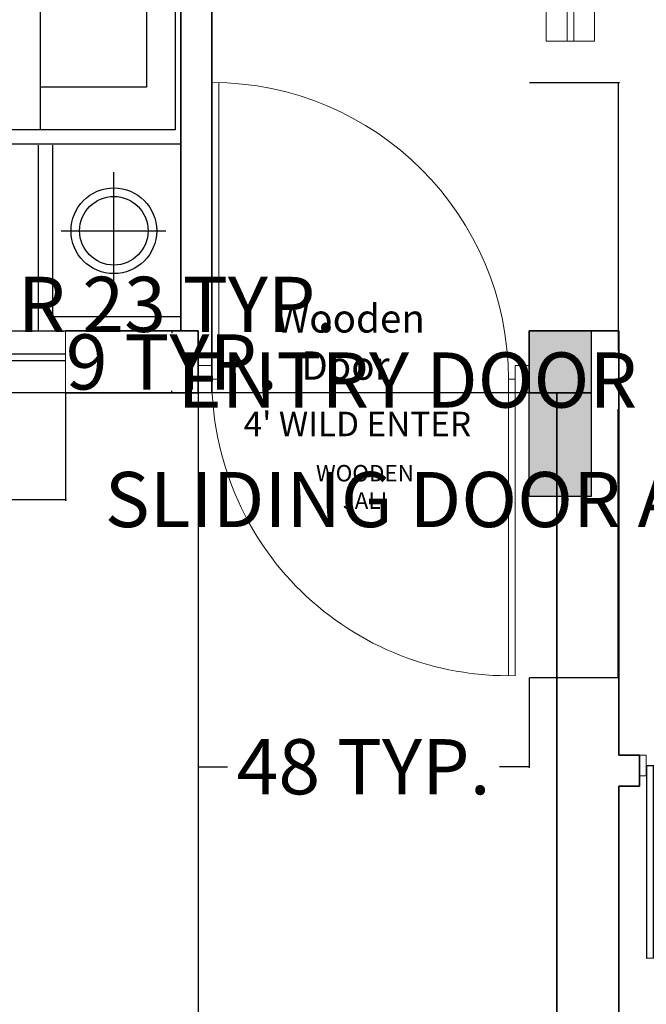
# Model space of a CAD drawing. Units: inches. Extents: x -48 to 50072, y 0 to 21068.
# Tile 61 of 75: x 883 to 974, y 660 to 803. Entities that reach past the tile are written whole.
import ezdxf

# ---------------------------------------------------------------- set-up
doc = ezdxf.new("R2010")
doc.units = ezdxf.units.IN
doc.header["$MEASUREMENT"] = 0
for name, color, linetype, lineweight in [('A-ANNO-DIMS', 2, 'Continuous', 18), ('A-ANNO-TEXT', 7, 'Continuous', 18), ('A-COLS', 1, 'Continuous', 35), ('A-DOOR', 4, 'Continuous', 18), ('A-FLOR-SCRN', 32, 'Continuous', 18), ('A-WALL', 7, 'Continuous', 35), ('FURNITURE', 44, 'Continuous', 18)]:
    doc.layers.add(name, color=color, linetype=linetype, lineweight=lineweight)
doc.layers.add('Layer3', color=176, linetype='Continuous')
doc.styles.get("Standard").update_dxf_attribs({"font": 'arial.ttf'})
doc.dimstyles.get("Standard").update_dxf_attribs({"dimtxt": 8, "dimasz": 0.18, "dimexe": 0.18, "dimexo": 0.0625, "dimgap": 0.09, "dimtad": 0, "dimtih": 1, "dimtoh": 1, "dimdec": 1, "dimzin": 0, "dimdsep": 46, "dimlunit": 4, "dimtxsty": 'Standard', "dimblk": 'ARCHTICK', "dimcen": 0.09, "dimadec": 0, "dimazin": 0, "dimtfac": 1, "dimtdec": 1, "dimtofl": 0, "dimtmove": 0, "dimatfit": 3, "dimldrblk": 'ARCHTICK', "dimfxl": 1, "dimtolj": 1, "dimtzin": 0, "dimarcsym": 0})

# ---------------------------------------------------------------- blocks, each defined once
blk = doc.blocks.new('bnniku')
at = {"layer": 'Defpoints'}
h = blk.add_hatch(color=256, dxfattribs=at)
h.dxf.hatch_style = 1
h.paths.add_polyline_path([(767.55, 1114.04), (758.55, 1114.04), (758.55, 1090.04), (767.55, 1090.04)])
for p, q in [((758.55, 1114.04), (767.55, 1114.04)), ((758.55, 1090.04), (758.55, 1114.04)), ((767.55, 1114.04), (767.55, 1090.04)), ((767.55, 1090.04), (758.55, 1090.04))]:
    blk.add_line(p, q, dxfattribs=at)
blk = doc.blocks.new('fdsghhhhhhygr')
for p, q in [((41.77, 686.77), (41.77, 677.77)), ((144.77, 677.77), (144.77, 686.77))]:
    blk.add_line(p, q)
at = {"layer": 'Defpoints'}
for p, q in [((91.27, 683.47), (144.77, 683.47)), ((91.27, 683.47), (91.27, 682.47)), ((91.27, 682.47), (144.77, 682.47)), ((41.77, 682.07), (95.27, 682.07)), ((41.77, 681.07), (95.27, 681.07)), ((95.27, 682.07), (95.27, 681.07))]:
    blk.add_line(p, q, dxfattribs=at)
at = {"layer": 'Layer3'}
for p, q in [((41.77, 686.77), (144.77, 686.77)), ((144.77, 677.77), (41.77, 677.77))]:
    blk.add_line(p, q, dxfattribs=at)
blk = doc.blocks.new('gthyerhy')
at = {"layer": 'Defpoints'}
for p, q in [((665.59, 603.33), (665.59, 631.33)), ((666.59, 603.33), (666.59, 631.32)), ((665.59, 603.33), (693.59, 603.33))]:
    blk.add_line(p, q, dxfattribs=at)
blk.add_arc((665.59, 603.33), 28, 0, 90, dxfattribs=at)
at = {"insert": (674.82, 600.63), "char_height": 2.3647, "attachment_point": 1}
blk.add_mtext_dynamic_manual_height_columns('\\pxqc;WOODEN ^JDOOR', width=6.8949, gutter_width=11.82, heights=[0], dxfattribs=at)
blk = doc.blocks.new('nhrygfdu7yu')
at = {"layer": 'Defpoints'}
for p, q in [((1019.17, 828.61), (845.97, 828.61)), ((845.97, 801.61), (845.97, 828.61)), ((848.67, 804.31), (848.67, 828.61)), ((881.27, 716.83), (881.27, 828.61)), ((983.87, 828.61), (983.87, 716.83)), ((1016.47, 804.31), (1016.47, 828.61)), ((1019.17, 801.61), (1019.17, 828.61)), ((884.03, 719.53), (884.03, 827.53)), ((884.03, 827.53), (981.17, 827.53)), ((981.17, 827.53), (981.17, 719.53)), ((864.18, 805.04), (864.18, 824.84)), ((1000.24, 805.98), (1000.24, 825.78)), ((892.12, 822.13), (892.12, 801.97)), ((929.67, 822.13), (892.12, 822.13)), ((929.67, 822.13), (929.67, 801.78)), ((935.52, 822.13), (935.52, 801.78)), ((935.52, 822.13), (973.07, 822.13)), ((973.07, 822.13), (973.07, 801.97)), ((926.47, 818.07), (927.21, 812.5)), ((947.88, 818.06), (943.61, 812.45)), ((1010.72, 815.93), (989.15, 815.93)), ((874.65, 814.99), (853.09, 814.99)), ((927.21, 812.5), (925.82, 805.91)), ((934.43, 807.75), (933.36, 812.55)), ((943.61, 812.45), (939.55, 805.41)), ((914.58, 810.18), (913.28, 809.99)), ((919.69, 808.14), (914.58, 810.18)), ((923.4, 803.12), (919.69, 808.14)), ((935.49, 804.66), (934.43, 807.75)), ((881.07, 804.31), (848.67, 804.31)), ((881.07, 804.31), (881.07, 804.31)), ((916.07, 804.42), (910.77, 803.49)), ((919.78, 804.61), (916.07, 804.42)), ((923.4, 803.12), (919.78, 804.61)), ((925.82, 805.91), (923.4, 803.12)), ((938.59, 802.42), (935.49, 804.66)), ((939.55, 805.41), (938.59, 802.42)), ((938.59, 802.42), (945.53, 804.13)), ((945.53, 804.13), (951.08, 803.38)), ((984.07, 804.31), (1016.47, 804.31)), ((984.07, 804.31), (984.07, 804.31)), ((910.77, 803.49), (910.59, 803.15)), ((923.4, 803.12), (925.08, 798.67)), ((923.4, 803.12), (933.44, 802.1)), ((935.45, 803.17), (936.69, 800.13)), ((938.59, 802.42), (937.95, 797.34)), ((938.59, 802.42), (941.26, 799.01)), ((951.08, 803.38), (953.02, 802.3)), ((881.07, 801.61), (845.97, 801.61)), ((884.06, 801.97), (981.18, 801.97)), ((933.44, 802.1), (936.13, 800.15)), ((984.07, 801.61), (1019.17, 801.61)), ((925.08, 798.67), (923.96, 794.21)), ((936.13, 800.15), (936.78, 799.69)), ((936.69, 800.13), (937.65, 797.78)), ((941.26, 799.01), (944.78, 796.45)), ((937.86, 796.54), (937.22, 791.44)), ((944.78, 796.45), (949.8, 796.45)), ((981.13, 793.06), (883.98, 783.7)), ((923.96, 794.21), (921.07, 790.83)), ((906.36, 766.47), (977.44, 792.73)), ((976.41, 779.36), (976.41, 779.36)), ((978.98, 779.36), (978.98, 779.36)), ((962.27, 776.79), (962.27, 776.79)), ((964.84, 776.79), (964.84, 776.79)), ((967.41, 776.79), (967.41, 776.79)), ((969.98, 776.79), (969.98, 776.79)), ((972.55, 776.79), (972.55, 776.79)), ((975.13, 776.79), (975.13, 776.79)), ((977.7, 776.79), (977.7, 776.79)), ((980.27, 776.79), (980.27, 776.79)), ((950.69, 774.21), (950.69, 774.21)), ((953.27, 774.21), (953.27, 774.21)), ((955.84, 774.21), (955.84, 774.21)), ((958.41, 774.21), (958.41, 774.21)), ((960.98, 774.21), (960.98, 774.21)), ((963.55, 774.21), (963.55, 774.21)), ((966.13, 774.21), (966.13, 774.21)), ((968.7, 774.21), (968.7, 774.21)), ((941.69, 771.64), (941.69, 771.64)), ((944.27, 771.64), (944.27, 771.64)), ((946.84, 771.64), (946.84, 771.64)), ((949.41, 771.64), (949.41, 771.64)), ((951.98, 771.64), (951.98, 771.64)), ((954.55, 771.64), (954.55, 771.64)), ((935.26, 769.07), (935.26, 769.07)), ((937.84, 769.07), (937.84, 769.07)), ((940.41, 769.07), (940.41, 769.07)), ((942.98, 769.07), (942.98, 769.07)), ((928.83, 766.5), (928.83, 766.5)), ((931.41, 766.5), (931.41, 766.5)), ((933.98, 766.5), (933.98, 766.5)), ((936.55, 766.5), (936.55, 766.5)), ((975.13, 766.5), (975.13, 766.5)), ((977.7, 766.5), (977.7, 766.5)), ((980.27, 766.5), (980.27, 766.5)), ((924.98, 763.93), (924.98, 763.93)), ((927.55, 763.93), (927.55, 763.93)), ((930.12, 763.93), (930.12, 763.93)), ((963.55, 763.93), (963.55, 763.93)), ((966.13, 763.93), (966.13, 763.93)), ((968.7, 763.93), (968.7, 763.93)), ((971.27, 763.93), (971.27, 763.93)), ((973.84, 763.93), (973.84, 763.93)), ((976.41, 763.93), (976.41, 763.93)), ((978.98, 763.93), (978.98, 763.93)), ((921.12, 761.35), (921.12, 761.35)), ((923.69, 761.35), (923.69, 761.35)), ((954.55, 761.35), (954.55, 761.35)), ((957.12, 761.35), (957.12, 761.35)), ((959.7, 761.35), (959.7, 761.35)), ((962.27, 761.35), (962.27, 761.35)), ((964.84, 761.35), (964.84, 761.35)), ((967.41, 761.35), (967.41, 761.35)), ((969.98, 761.35), (969.98, 761.35)), ((972.55, 761.35), (972.55, 761.35)), ((975.13, 761.35), (975.13, 761.35)), ((917.26, 758.78), (917.26, 758.78)), ((919.83, 758.78), (919.83, 758.78)), ((945.55, 758.78), (945.55, 758.78)), ((948.12, 758.78), (948.12, 758.78)), ((950.69, 758.78), (950.69, 758.78)), ((953.27, 758.78), (953.27, 758.78)), ((955.84, 758.78), (955.84, 758.78)), ((958.41, 758.78), (958.41, 758.78)), ((960.98, 758.78), (960.98, 758.78)), ((963.55, 758.78), (963.55, 758.78)), ((913.4, 756.21), (913.4, 756.21)), ((915.98, 756.21), (915.98, 756.21)), ((941.69, 756.21), (941.69, 756.21)), ((944.27, 756.21), (944.27, 756.21)), ((946.84, 756.21), (946.84, 756.21)), ((949.41, 756.21), (949.41, 756.21)), ((951.98, 756.21), (951.98, 756.21)), ((954.55, 756.21), (954.55, 756.21)), ((957.12, 756.21), (957.12, 756.21)), ((980.27, 756.21), (980.27, 756.21)), ((909.55, 753.64), (909.55, 753.64)), ((912.12, 753.64), (912.12, 753.64)), ((935.26, 753.64), (935.26, 753.64)), ((937.84, 753.64), (937.84, 753.64)), ((940.41, 753.64), (940.41, 753.64)), ((942.98, 753.64), (942.98, 753.64)), ((945.55, 753.64), (945.55, 753.64)), ((948.12, 753.64), (948.12, 753.64)), ((976.41, 753.64), (976.41, 753.64)), ((978.98, 753.64), (978.98, 753.64)), ((905.69, 751.07), (905.69, 751.07)), ((908.26, 751.07), (908.26, 751.07)), ((931.41, 751.07), (931.41, 751.07)), ((933.98, 751.07), (933.98, 751.07)), ((936.55, 751.07), (936.55, 751.07)), ((939.12, 751.07), (939.12, 751.07)), ((941.69, 751.07), (941.69, 751.07)), ((944.27, 751.07), (944.27, 751.07)), ((969.98, 751.07), (969.98, 751.07)), ((972.55, 751.07), (972.55, 751.07)), ((975.13, 751.07), (975.13, 751.07)), ((977.7, 751.07), (977.7, 751.07)), ((980.27, 751.07), (980.27, 751.07)), ((904.4, 748.5), (904.4, 748.5)), ((927.55, 748.5), (927.55, 748.5)), ((930.12, 748.5), (930.12, 748.5)), ((932.69, 748.5), (932.69, 748.5)), ((935.26, 748.5), (935.26, 748.5)), ((937.84, 748.5), (937.84, 748.5)), ((940.41, 748.5), (940.41, 748.5)), ((966.13, 748.5), (966.13, 748.5)), ((968.7, 748.5), (968.7, 748.5)), ((971.27, 748.5), (971.27, 748.5)), ((973.84, 748.5), (973.84, 748.5)), ((976.41, 748.5), (976.41, 748.5)), ((978.98, 748.5), (978.98, 748.5)), ((900.55, 745.92), (900.55, 745.92)), ((903.12, 745.92), (903.12, 745.92)), ((923.69, 745.92), (923.69, 745.92)), ((926.26, 745.92), (926.26, 745.92)), ((928.83, 745.92), (928.83, 745.92)), ((931.41, 745.92), (931.41, 745.92)), ((933.98, 745.92), (933.98, 745.92)), ((962.27, 745.92), (962.27, 745.92)), ((964.84, 745.92), (964.84, 745.92)), ((967.41, 745.92), (967.41, 745.92)), ((969.98, 745.92), (969.98, 745.92)), ((972.55, 745.92), (972.55, 745.92)), ((975.13, 745.92), (975.13, 745.92)), ((977.7, 745.92), (977.7, 745.92)), ((896.69, 743.35), (896.69, 743.35)), ((899.26, 743.35), (899.26, 743.35)), ((919.83, 743.35), (919.83, 743.35)), ((922.41, 743.35), (922.41, 743.35)), ((924.98, 743.35), (924.98, 743.35)), ((927.55, 743.35), (927.55, 743.35)), ((930.12, 743.35), (930.12, 743.35)), ((932.69, 743.35), (932.69, 743.35)), ((960.98, 743.35), (960.98, 743.35)), ((963.55, 743.35), (963.55, 743.35)), ((966.13, 743.35), (966.13, 743.35)), ((968.7, 743.35), (968.7, 743.35)), ((971.27, 743.35), (971.27, 743.35)), ((973.84, 743.35), (973.84, 743.35)), ((895.4, 740.78), (895.4, 740.78)), ((915.98, 740.78), (915.98, 740.78)), ((918.55, 740.78), (918.55, 740.78)), ((921.12, 740.78), (921.12, 740.78)), ((923.69, 740.78), (923.69, 740.78)), ((926.26, 740.78), (926.26, 740.78)), ((928.83, 740.78), (928.83, 740.78)), ((957.12, 740.78), (957.12, 740.78)), ((959.7, 740.78), (959.7, 740.78)), ((962.27, 740.78), (962.27, 740.78)), ((964.84, 740.78), (964.84, 740.78)), ((967.41, 740.78), (967.41, 740.78)), ((969.98, 740.78), (969.98, 740.78)), ((891.54, 738.21), (891.54, 738.21)), ((894.12, 738.21), (894.12, 738.21)), ((914.69, 738.21), (914.69, 738.21)), ((917.26, 738.21), (917.26, 738.21)), ((919.83, 738.21), (919.83, 738.21)), ((922.41, 738.21), (922.41, 738.21)), ((924.98, 738.21), (924.98, 738.21)), ((955.84, 738.21), (955.84, 738.21)), ((958.41, 738.21), (958.41, 738.21)), ((960.98, 738.21), (960.98, 738.21)), ((963.55, 738.21), (963.55, 738.21)), ((966.13, 738.21), (966.13, 738.21)), ((887.69, 735.64), (887.69, 735.64)), ((890.26, 735.64), (890.26, 735.64)), ((910.83, 735.64), (910.83, 735.64)), ((913.4, 735.64), (913.4, 735.64)), ((915.98, 735.64), (915.98, 735.64)), ((918.55, 735.64), (918.55, 735.64)), ((921.12, 735.64), (921.12, 735.64)), ((951.98, 735.64), (951.98, 735.64)), ((954.55, 735.64), (954.55, 735.64)), ((957.12, 735.64), (957.12, 735.64)), ((959.7, 735.64), (959.7, 735.64)), ((962.27, 735.64), (962.27, 735.64)), ((964.84, 735.64), (964.84, 735.64)), ((886.4, 733.07), (886.4, 733.07)), ((888.97, 733.07), (888.97, 733.07)), ((909.55, 733.07), (909.55, 733.07)), ((912.12, 733.07), (912.12, 733.07)), ((914.69, 733.07), (914.69, 733.07)), ((917.26, 733.07), (917.26, 733.07)), ((919.83, 733.07), (919.83, 733.07)), ((950.69, 733.07), (950.69, 733.07)), ((953.27, 733.07), (953.27, 733.07)), ((955.84, 733.07), (955.84, 733.07)), ((958.41, 733.07), (958.41, 733.07)), ((960.98, 733.07), (960.98, 733.07)), ((885.12, 730.49), (885.12, 730.49)), ((905.69, 730.49), (905.69, 730.49)), ((908.26, 730.49), (908.26, 730.49)), ((910.83, 730.49), (910.83, 730.49)), ((913.4, 730.49), (913.4, 730.49)), ((915.98, 730.49), (915.98, 730.49)), ((946.84, 730.49), (946.84, 730.49)), ((949.41, 730.49), (949.41, 730.49)), ((951.98, 730.49), (951.98, 730.49)), ((954.55, 730.49), (954.55, 730.49)), ((957.12, 730.49), (957.12, 730.49)), ((959.7, 730.49), (959.7, 730.49)), ((904.4, 727.92), (904.4, 727.92)), ((906.97, 727.92), (906.97, 727.92)), ((909.55, 727.92), (909.55, 727.92)), ((912.12, 727.92), (912.12, 727.92)), ((945.55, 727.92), (945.55, 727.92)), ((948.12, 727.92), (948.12, 727.92)), ((950.69, 727.92), (950.69, 727.92)), ((953.27, 727.92), (953.27, 727.92)), ((955.84, 727.92), (955.84, 727.92)), ((958.41, 727.92), (958.41, 727.92)), ((900.55, 725.35), (900.55, 725.35)), ((903.12, 725.35), (903.12, 725.35)), ((905.69, 725.35), (905.69, 725.35)), ((908.26, 725.35), (908.26, 725.35)), ((910.83, 725.35), (910.83, 725.35)), ((944.27, 725.35), (944.27, 725.35)), ((946.84, 725.35), (946.84, 725.35)), ((949.41, 725.35), (949.41, 725.35)), ((951.98, 725.35), (951.98, 725.35)), ((954.55, 725.35), (954.55, 725.35)), ((899.26, 722.78), (899.26, 722.78)), ((901.83, 722.78), (901.83, 722.78)), ((904.4, 722.78), (904.4, 722.78)), ((906.97, 722.78), (906.97, 722.78)), ((942.98, 722.78), (942.98, 722.78)), ((945.55, 722.78), (945.55, 722.78)), ((948.12, 722.78), (948.12, 722.78)), ((950.69, 722.78), (950.69, 722.78)), ((953.27, 722.78), (953.27, 722.78)), ((981.17, 719.53), (884.03, 719.53)), ((895.4, 720.21), (895.4, 720.21)), ((897.97, 720.21), (897.97, 720.21)), ((900.55, 720.21), (900.55, 720.21)), ((903.12, 720.21), (903.12, 720.21)), ((905.69, 720.21), (905.69, 720.21)), ((939.12, 720.21), (939.12, 720.21)), ((941.69, 720.21), (941.69, 720.21)), ((944.27, 720.21), (944.27, 720.21)), ((946.84, 720.21), (946.84, 720.21)), ((949.41, 720.21), (949.41, 720.21)), ((951.98, 720.21), (951.98, 720.21)), ((983.87, 716.83), (881.27, 716.83))]:
    blk.add_line(p, q, dxfattribs=at)
for centre, radius in [((864.18, 814.99), 8.1), ((1000.24, 815.93), 8.1), ((864.18, 814.99), 6.48), ((1000.24, 815.93), 6.48)]:
    blk.add_circle(centre, radius, dxfattribs=at)
for centre, radius, start, end in [((924.05, 817.43), 1.94, 297.2902, 3.2455), ((926.67, 817.58), 0.687, 51.1864, 183.2455), ((924.75, 815.18), 3.76, 45.8726, 51.1864), ((929.07, 819.63), 2.44, 225.8726, 232.4713), ((940.16, 834.08), 20.66, 232.4713, 233.7837), ((906.88, 788.64), 35.67, 52.7849, 53.7837), ((943.53, 820.78), 4.28, 292.7069, 308.5854), ((948.22, 814.9), 3.25, 110.3452, 128.5854), ((947.75, 816.16), 1.9, 86.0516, 110.3452), ((948.43, 816.91), 0.765, 126.5792, 169.5926), ((947.87, 817.82), 0.239, 13.2808, 86.0516), ((947.77, 817.8), 0.34, 306.5792, 13.2808), ((848.26, 964.34), 167.25, 296.4147, 297.2902), ((921.35, 807.68), 11.75, 46.4776, 52.7849), ((926.56, 813.17), 4.18, 35.8936, 46.4776), ((928.96, 814.91), 1.22, 351.9508, 35.8936), ((848.62, 1074.38), 275.09, 289.0836, 290.1287), ((927.73, 858.54), 45.2, 290.1287, 292.7069), ((951.77, 816.3), 4.17, 169.5926, 177.2714), ((948.44, 816.46), 0.826, 177.2714, 194.5709), ((949.69, 816.78), 2.12, 194.5709, 206.8179), ((964.76, 824.4), 19.01, 206.8179, 210.9056), ((1072.97, 521.35), 329.5, 117.4999, 117.8482), ((971.1, 717.04), 108.88, 116.4147, 117.4999), ((932.62, 814.39), 2.47, 171.9508, 202.4162), ((980.52, 834.15), 54.29, 202.4162, 205.0529), ((883.03, 974.91), 169.83, 286.6085, 289.0836), ((957.44, 820.02), 10.47, 210.9056, 219.7005), ((901.77, 841.65), 33.68, 290.7486, 297.4921), ((771.78, 1091.44), 315.27, 297.4921, 297.8482), ((929.77, 818.2), 6.29, 280.7366, 286.6085), ((946.01, 810.53), 4.37, 26.0735, 39.7005), ((940.41, 807.79), 10.61, 17.8396, 26.0735), ((905.47, 831.87), 23.22, 282.6252, 290.7486), ((1013.86, 849.73), 91.09, 205.0529, 207.0884), ((847.55, 777.91), 108.16, 15.2625, 17.8396), ((908.02, 808.45), 0.313, 121.6917, 179.0386), ((908.61, 808.44), 0.905, 179.0386, 229.4914), ((909.3, 806.38), 2.75, 103.0402, 121.6917), ((909.41, 805.91), 3.23, 86.6119, 103.0402), ((909.8, 812.53), 3.4, 266.6119, 282.6252), ((1008.01, 846.74), 84.52, 207.0884, 209.936), ((905.38, 804.66), 4.08, 26.3332, 49.4914), ((780.21, 742.7), 143.74, 25.1732, 26.3332), ((866.04, 782.95), 89, 13.841, 15.2625), ((924.73, 798.79), 11.57, 22.2355, 29.936), ((981.05, 811.29), 29.45, 193.841, 196.3122), ((901.51, 799.71), 9.71, 20.7081, 25.1732), ((883.04, 792.73), 29.45, 18.2369, 20.7081), ((962.1, 805.74), 9.71, 196.3122, 200.7773), ((1087.42, 853.29), 143.74, 200.7773, 201.9373), ((995.54, 829.8), 89, 198.2369, 199.6584), ((1013.59, 836.25), 108.16, 199.6584, 202.2355), ((957.87, 801.11), 4.08, 201.9373, 225.0955), ((938.8, 798.25), 1.24, 202.2355, 252.8133), ((938.36, 796.82), 0.252, 289.3799, 72.8133), ((955.69, 773.98), 23.22, 98.2293, 106.3527), ((952.85, 793.6), 3.4, 82.216, 98.2293), ((953.75, 800.17), 3.23, 262.216, 278.6443), ((953.82, 799.69), 2.75, 278.6443, 297.2959), ((954.35, 797.58), 0.905, 354.6428, 45.0955), ((954.94, 797.53), 0.313, 297.2959, 354.6428), ((923.29, 799.33), 10.61, 202.2355, 210.4694), ((993.31, 637.11), 169.83, 111.0043, 113.4795), ((880.68, 777.46), 54.29, 18.0203, 19.3448), ((934.7, 789.77), 6.29, 98.1216, 111.0043), ((934.31, 792.46), 3.58, 85.4882, 98.1216), ((934.9, 799.87), 3.85, 265.4882, 277.6784), ((934.12, 805.65), 9.69, 277.6784, 284.8807), ((939.32, 786.09), 10.56, 97.9822, 104.8807), ((938.1, 794.73), 1.83, 85.7407, 97.9822), ((938.28, 797.05), 0.497, 265.7407, 289.3799), ((1069.09, 504.93), 315.27, 113.0962, 113.4523), ((958.63, 763.95), 33.68, 106.3527, 113.0962), ((917.92, 796.17), 4.37, 210.4694, 224.0964), ((907.26, 785.84), 10.47, 35.3015, 44.0964), ((929.96, 793.49), 2.47, 347.5549, 18.0203), ((933.57, 792.7), 1.22, 167.5549, 211.4977), ((899.06, 893.51), 108.88, 292.0188, 293.104), ((812.48, 1096.43), 329.5, 293.104, 293.4523), ((900.29, 780.91), 19.01, 31.2138, 35.3015), ((1035.25, 540.56), 275.09, 113.4795, 114.5246), ((936.09, 794.24), 4.18, 211.4977, 222.0817), ((941.71, 799.32), 11.75, 222.0817, 228.389), ((938.27, 789.81), 1.94, 112.8944, 178.8496), ((1002.58, 637.52), 167.25, 112.0188, 112.8944), ((916, 789.63), 0.765, 310.9751, 353.9885), ((914.73, 789.66), 2.12, 18.9668, 31.2138), ((915.96, 790.08), 0.826, 1.6673, 18.9668), ((912.62, 789.98), 4.17, 353.9885, 1.6673), ((916.05, 791.65), 3.25, 294.7411, 312.9813), ((921.18, 786.14), 4.28, 117.1028, 132.9813), ((939.83, 749.71), 45.2, 114.5246, 117.1028), ((957.59, 817.2), 35.67, 228.389, 229.3878), ((920.93, 774.44), 20.66, 48.0754, 49.3878), ((933.1, 787.99), 2.44, 41.4767, 48.0754), ((937.75, 792.1), 3.76, 221.4767, 226.7905), ((935.64, 789.86), 0.687, 226.7905, 358.8496), ((916.73, 788.79), 0.34, 130.9751, 197.6767), ((916.63, 788.76), 0.239, 197.6767, 270.4475), ((916.62, 790.42), 1.9, 270.4475, 294.7411)]:
    blk.add_arc(centre, radius, start, end, dxfattribs=at)
blk.add_ellipse((874.1, 762.91), major_axis=(32.71, 0), ratio=0.667085, start_param=0.16392, end_param=1.263761, dxfattribs=at)
blk = doc.blocks.new('DOOR-ENTRY-TANDEM-48')
for p, q in [((2, 43), (2, 86)), ((3, 85.99), (3, 43)), ((0, 45), (2, 45)), ((2, 41), (2, 45)), ((46, 41), (46, 45)), ((46, 45), (48, 45)), ((2, 43), (3, 43)), ((2, 43), (3, 43)), ((2, 43), (3, 43)), ((45, 0), (45, 43)), ((45, 43), (46, 43)), ((46, 43), (46, 7)), ((0, 41), (48, 41)), ((46, 7), (46, 0.01))]:
    blk.add_line(p, q)
for centre, start, end in [((2, 43), 0, 90), ((45, 43), 180, 271.3326)]:
    blk.add_arc(centre, 43, start, end)
blk = doc.blocks.new('SCREEN-JALI-90')
for p, q in [((7, 90), (0, 90)), ((0, 90), (0, 0)), ((3, 90), (3, 0)), ((4, 90), (4, 0)), ((7, 0), (7, 90)), ((7, 0), (0, 0))]:
    blk.add_line(p, q)
blk = doc.blocks.new('_ArchTick')
at = {"color": 0, "linetype": 'ByBlock', "const_width": 0.15}
blk.add_lwpolyline([(-0.5, -0.5), (0.5, 0.5)], dxfattribs=at)
blk = doc.blocks.new('*D60')
at = {"layer": 'A-ANNO-DIMS', "color": 0, "lineweight": -2, "transparency": 16777216}
for p, q in [((787.01, 748.4), (787.01, 732.83)), ((890.01, 748.4), (890.01, 732.83)), ((787.01, 733.01), (890.01, 733.01)), ((890.01, 733.01), (890.19, 733.01))]:
    blk.add_line(p, q, dxfattribs=at)
at = {"layer": 'Defpoints', "color": 0, "transparency": 16777216}
for p in [(787.01, 748.46), (890.01, 748.46), (890.01, 733.01)]:
    blk.add_point(p, dxfattribs=at)
at = {"layer": 'A-ANNO-DIMS', "color": 0, "lineweight": -2, "transparency": 16777216, "xscale": 0.18, "yscale": 0.18, "zscale": 0.18, "rotation": 180}
blk.add_blockref('_ArchTick', (787.01, 733.01), dxfattribs=at)
at = {"layer": 'A-ANNO-DIMS', "color": 0, "lineweight": -2, "transparency": 16777216, "xscale": 0.18, "yscale": 0.18, "zscale": 0.18}
blk.add_blockref('_ArchTick', (890.01, 733.01), dxfattribs=at)
at = {"layer": 'A-ANNO-DIMS', "color": 0, "transparency": 16777216, "insert": (960.35, 733.01), "char_height": 8, "attachment_point": 5}
blk.add_mtext('\\A1;SLIDING DOOR A 103 TYP.', dxfattribs=at)
blk = doc.blocks.new('*D61')
at = {"layer": 'A-ANNO-DIMS', "color": 0, "lineweight": -2, "transparency": 16777216}
for p, q in [((890.07, 757.46), (905.64, 757.46)), ((905.46, 757.46), (905.46, 757.14)), ((890.07, 748.46), (905.64, 748.46)), ((905.46, 748.46), (905.46, 748.79))]:
    blk.add_line(p, q, dxfattribs=at)
at = {"layer": 'Defpoints', "color": 0, "transparency": 16777216}
for p in [(890.01, 757.46), (905.46, 757.46), (890.01, 748.46)]:
    blk.add_point(p, dxfattribs=at)
at = {"layer": 'A-ANNO-DIMS', "color": 0, "lineweight": -2, "transparency": 16777216, "xscale": 0.18, "yscale": 0.18, "zscale": 0.18}
for p, rotation in [((905.46, 757.46), 90), ((905.46, 748.46), 270)]:
    blk.add_blockref('_ArchTick', p, dxfattribs=dict(at, rotation=rotation))
at = {"layer": 'A-ANNO-DIMS', "color": 0, "transparency": 16777216, "insert": (905.46, 752.96), "char_height": 8, "attachment_point": 5}
blk.add_mtext('\\A1;9 TYP.', dxfattribs=at)
blk = doc.blocks.new('*D76')
at = {"layer": 'A-ANNO-DIMS', "color": 0, "lineweight": -2, "transparency": 16777216}
for p, q in [((972.12, 817.98), (972.12, 806.85)), ((1045.51, 817.98), (1045.51, 806.85)), ((972.12, 807.03), (1045.51, 807.03)), ((1045.51, 807.03), (1045.69, 807.03))]:
    blk.add_line(p, q, dxfattribs=at)
at = {"layer": 'Defpoints', "color": 0, "transparency": 16777216}
for p in [(972.12, 818.04), (1045.51, 818.04), (1045.51, 807.03)]:
    blk.add_point(p, dxfattribs=at)
at = {"layer": 'A-ANNO-DIMS', "color": 0, "lineweight": -2, "transparency": 16777216, "xscale": 0.18, "yscale": 0.18, "zscale": 0.18, "rotation": 180}
blk.add_blockref('_ArchTick', (972.12, 807.03), dxfattribs=at)
at = {"layer": 'A-ANNO-DIMS', "color": 0, "lineweight": -2, "transparency": 16777216, "xscale": 0.18, "yscale": 0.18, "zscale": 0.18}
blk.add_blockref('_ArchTick', (1045.51, 807.03), dxfattribs=at)
at = {"layer": 'A-ANNO-DIMS', "color": 0, "transparency": 16777216, "insert": (1102.65, 807.03), "char_height": 8, "attachment_point": 5}
blk.add_mtext('\\A1;LOUNGE SET 73 TYP.', dxfattribs=at)
blk = doc.blocks.new('*D80')
at = {"layer": 'A-ANNO-DIMS', "color": 0, "lineweight": -2, "transparency": 16777216}
for p, q in [((793.35, 764.7), (793.35, 761.13)), ((816.36, 764.7), (816.36, 761.13)), ((793.35, 761.31), (816.36, 761.31)), ((816.36, 761.31), (816.54, 761.31))]:
    blk.add_line(p, q, dxfattribs=at)
at = {"layer": 'Defpoints', "color": 0, "transparency": 16777216}
for p in [(793.35, 764.76), (816.36, 764.76), (816.36, 761.31)]:
    blk.add_point(p, dxfattribs=at)
at = {"layer": 'A-ANNO-DIMS', "color": 0, "lineweight": -2, "transparency": 16777216, "xscale": 0.18, "yscale": 0.18, "zscale": 0.18, "rotation": 180}
blk.add_blockref('_ArchTick', (793.35, 761.31), dxfattribs=at)
at = {"layer": 'A-ANNO-DIMS', "color": 0, "lineweight": -2, "transparency": 16777216, "xscale": 0.18, "yscale": 0.18, "zscale": 0.18}
blk.add_blockref('_ArchTick', (816.36, 761.31), dxfattribs=at)
at = {"layer": 'A-ANNO-DIMS', "color": 0, "transparency": 16777216, "insert": (875.51, 761.31), "char_height": 8, "attachment_point": 5}
blk.add_mtext('\\A1;STUDY CHAIR 23 TYP.', dxfattribs=at)
blk = doc.blocks.new('*D98')
at = {"layer": 'A-ANNO-DIMS', "color": 0, "lineweight": -2, "transparency": 16777216}
for p, q in [((957.32, 793.46), (970.38, 793.46)), ((970.2, 793.46), (970.2, 754.56)), ((970.2, 707.21), (970.2, 746.11)), ((957.32, 707.21), (970.38, 707.21))]:
    blk.add_line(p, q, dxfattribs=at)
at = {"layer": 'Defpoints', "color": 0, "transparency": 16777216}
for p in [(957.26, 793.46), (970.2, 793.46), (957.26, 707.21)]:
    blk.add_point(p, dxfattribs=at)
at = {"layer": 'A-ANNO-DIMS', "color": 0, "lineweight": -2, "transparency": 16777216, "xscale": 0.18, "yscale": 0.18, "zscale": 0.18}
for p, rotation in [((970.2, 793.46), 90), ((970.2, 707.21), 270)]:
    blk.add_blockref('_ArchTick', p, dxfattribs=dict(at, rotation=rotation))
at = {"layer": 'A-ANNO-DIMS', "color": 0, "transparency": 16777216, "insert": (970.2, 750.34), "char_height": 8, "attachment_point": 5}
blk.add_mtext('\\A1;ENTRY DOOR SET 86 TYP.', dxfattribs=at)
blk = doc.blocks.new('*D99')
at = {"layer": 'A-ANNO-DIMS', "color": 0, "lineweight": -2, "transparency": 16777216}
for p, q in [((909.26, 707.14), (909.26, 694.09)), ((957.26, 707.14), (957.26, 694.09)), ((909.26, 694.27), (913.54, 694.27)), ((957.26, 694.27), (952.98, 694.27))]:
    blk.add_line(p, q, dxfattribs=at)
at = {"layer": 'Defpoints', "color": 0, "transparency": 16777216}
for p in [(909.26, 707.21), (957.26, 707.21), (957.26, 694.27)]:
    blk.add_point(p, dxfattribs=at)
at = {"layer": 'A-ANNO-DIMS', "color": 0, "lineweight": -2, "transparency": 16777216, "xscale": 0.18, "yscale": 0.18, "zscale": 0.18, "rotation": 180}
blk.add_blockref('_ArchTick', (909.26, 694.27), dxfattribs=at)
at = {"layer": 'A-ANNO-DIMS', "color": 0, "lineweight": -2, "transparency": 16777216, "xscale": 0.18, "yscale": 0.18, "zscale": 0.18}
blk.add_blockref('_ArchTick', (957.26, 694.27), dxfattribs=at)
at = {"layer": 'A-ANNO-DIMS', "color": 0, "transparency": 16777216, "insert": (933.26, 694.27), "char_height": 8, "attachment_point": 5}
blk.add_mtext('\\A1;48 TYP.', dxfattribs=at)
blk = doc.blocks.new('*D135')
at = {"layer": 'A-ANNO-DIMS', "color": 0, "lineweight": -2, "transparency": 16777216}
for p, q in [((763.26, 748.4), (763.26, 236.63)), ((909.26, 748.4), (909.26, 236.63)), ((763.26, 236.81), (827.71, 236.81)), ((909.26, 236.81), (844.81, 236.81))]:
    blk.add_line(p, q, dxfattribs=at)
at = {"layer": 'Defpoints', "color": 0, "transparency": 16777216}
for p in [(763.26, 748.46), (909.26, 748.46), (909.26, 236.81)]:
    blk.add_point(p, dxfattribs=at)
at = {"layer": 'A-ANNO-DIMS', "color": 0, "lineweight": -2, "transparency": 16777216, "xscale": 0.18, "yscale": 0.18, "zscale": 0.18, "rotation": 180}
blk.add_blockref('_ArchTick', (763.26, 236.81), dxfattribs=at)
at = {"layer": 'A-ANNO-DIMS', "color": 0, "lineweight": -2, "transparency": 16777216, "xscale": 0.18, "yscale": 0.18, "zscale": 0.18}
blk.add_blockref('_ArchTick', (909.26, 236.81), dxfattribs=at)
at = {"layer": 'A-ANNO-DIMS', "color": 0, "transparency": 16777216, "insert": (836.26, 236.81), "char_height": 8, "attachment_point": 5}
blk.add_mtext('\\A1;146', dxfattribs=at)
blk = doc.blocks.new('*D136')
at = {"layer": 'A-ANNO-DIMS', "color": 0, "lineweight": -2, "transparency": 16777216}
for p, q in [((909.26, 748.4), (909.26, 236.63)), ((961.26, 559.4), (961.26, 236.63)), ((909.26, 236.81), (929.48, 236.81)), ((961.26, 236.81), (941.04, 236.81))]:
    blk.add_line(p, q, dxfattribs=at)
at = {"layer": 'Defpoints', "color": 0, "transparency": 16777216}
for p in [(909.26, 748.46), (961.26, 559.46), (961.26, 236.81)]:
    blk.add_point(p, dxfattribs=at)
at = {"layer": 'A-ANNO-DIMS', "color": 0, "lineweight": -2, "transparency": 16777216, "xscale": 0.18, "yscale": 0.18, "zscale": 0.18, "rotation": 180}
blk.add_blockref('_ArchTick', (909.26, 236.81), dxfattribs=at)
at = {"layer": 'A-ANNO-DIMS', "color": 0, "lineweight": -2, "transparency": 16777216, "xscale": 0.18, "yscale": 0.18, "zscale": 0.18}
blk.add_blockref('_ArchTick', (961.26, 236.81), dxfattribs=at)
at = {"layer": 'A-ANNO-DIMS', "color": 0, "transparency": 16777216, "insert": (935.26, 236.81), "char_height": 8, "attachment_point": 5}
blk.add_mtext('\\A1;52', dxfattribs=at)
blk = doc.blocks.new('*D145')
at = {"layer": 'A-ANNO-DIMS', "color": 0, "lineweight": -2, "transparency": 16777216}
for p, q in [((961.2, 748.46), (710.63, 748.46)), ((710.81, 748.46), (710.81, 658.14)), ((710.81, 559.46), (710.81, 649.79)), ((961.2, 559.46), (710.63, 559.46))]:
    blk.add_line(p, q, dxfattribs=at)
at = {"layer": 'Defpoints', "color": 0, "transparency": 16777216}
for p in [(710.81, 748.46), (961.26, 748.46), (961.26, 559.46)]:
    blk.add_point(p, dxfattribs=at)
at = {"layer": 'A-ANNO-DIMS', "color": 0, "lineweight": -2, "transparency": 16777216, "xscale": 0.18, "yscale": 0.18, "zscale": 0.18}
for p, rotation in [((710.81, 748.46), 90), ((710.81, 559.46), 270)]:
    blk.add_blockref('_ArchTick', p, dxfattribs=dict(at, rotation=rotation))
at = {"layer": 'A-ANNO-DIMS', "color": 0, "transparency": 16777216, "insert": (710.81, 653.96), "char_height": 8, "attachment_point": 5}
blk.add_mtext('\\A1;189', dxfattribs=at)

msp = doc.modelspace()

# ---------------------------------------------------------------- linework, layer by layer
at = {"layer": 'A-DOOR'}
for p, q in [((973.261, 695.964), (974.261, 695.964)), ((974.261, 692.964), (974.261, 695.964)), ((973.261, 692.964), (974.261, 692.964))]:
    msp.add_line(p, q, dxfattribs=at)
at = {"layer": 'A-WALL'}
for p, q in [((906.761, 931.464), (906.761, 757.464)), ((911.261, 931.464), (911.261, 748.464)), ((909.261, 757.464), (890.012, 757.464)), ((909.261, 748.464), (909.261, 757.464)), ((957.261, 748.464), (957.261, 757.464)), ((970.261, 757.464), (957.261, 757.464)), ((970.261, 695.964), (970.261, 757.464)), ((909.261, 748.464), (890.012, 748.464)), ((966.261, 748.464), (957.261, 748.464)), ((961.261, 559.464), (961.261, 748.464)), ((973.261, 695.964), (970.261, 695.964)), ((973.261, 691.464), (973.261, 695.964)), ((970.261, 568.464), (970.261, 691.464)), ((973.261, 691.464), (970.261, 691.464))]:
    msp.add_line(p, q, dxfattribs=at)

# ---------------------------------------------------------------- block references
at = {"layer": 'A-COLS'}
msp.add_blockref('bnniku', (198.709, -356.573), dxfattribs=at)
at = {"layer": 'A-DOOR'}
for name, p in [('DOOR-ENTRY-TANDEM-48', (909.261, 707.464)), ('fdsghhhhhhygr', (745.244, 70.689))]:
    msp.add_blockref(name, p, dxfattribs=at)
at = {"layer": 'A-DOOR', "xscale": -1, "rotation": 180}
msp.add_blockref('gthyerhy', (308.676, 1297.798), dxfattribs=at)
at = {"layer": 'A-FLOR-SCRN'}
msp.add_blockref('SCREEN-JALI-90', (959.761, 799.464), dxfattribs=at)
at = {"layer": 'FURNITURE', "xscale": 0.7669307891904348, "yscale": 0.7669307891904348, "zscale": 0.7669307891904348, "rotation": 270}
msp.add_blockref('nhrygfdu7yu', (271.278, 1539.095), dxfattribs=at)

# ---------------------------------------------------------------- texts
at = {"layer": 'A-ANNO-TEXT', "attachment_point": 1}
for s, width, gutter_width, insert, char_height in [('Wooden^J   Door', 42.42894, 20.514, (920.464, 761.322), 4.10286), ("4' WILD ENTER", 45.36164, 17.739, (915.86, 745.739), 3.5477), ('\\pxqc;WOODEN^JJALI', 27.24055, 11.943, (919.835, 738.021), 2.38857)]:
    msp.add_mtext_dynamic_manual_height_columns(s, width=width, gutter_width=gutter_width, heights=[0], dxfattribs=dict(at, insert=insert, char_height=char_height))

# ---------------------------------------------------------------- dimensions: what is measured, and where the dimension line sits
at = {"layer": 'A-ANNO-DIMS'}
for base, p1, p2, text, picture, middle in [((1045.513, 807.034), (972.121, 818.043), (1045.513, 818.043), 'LOUNGE SET <> TYP.', '*D76', (1102.648, 807.034)), ((816.358, 761.309), (793.355, 764.76), (816.358, 764.76), 'STUDY CHAIR <> TYP.', '*D80', (875.509, 761.309)), ((890.012, 733.014), (787.01, 748.464), (890.012, 748.464), 'SLIDING DOOR A <> TYP.', '*D60', (960.347, 733.014)), ((957.261, 694.268), (909.261, 707.206), (957.261, 707.206), '<> TYP.', '*D99', (933.261, 694.268))]:
    dim = msp.add_linear_dim(base=base, p1=p1, p2=p2, text=text, dimstyle='Standard', override={"dimdec": 0, "dimlfac": 1, "dimrnd": 0, "dimzin": 0, "dimdsep": 46, "dimlunit": 2}, dxfattribs=at)
    dim.commit()
    dim.dimension.update_dxf_attribs({"geometry": picture, "text_midpoint": middle})
for base, p1, p2, text, picture, middle in [((970.199, 793.464), (957.261, 707.206), (957.261, 793.464), 'ENTRY DOOR SET <> TYP.', '*D98', (970.199, 750.335)), ((905.462, 757.464), (890.012, 748.464), (890.012, 757.464), '<> TYP.', '*D61', (905.462, 752.964))]:
    dim = msp.add_linear_dim(base=base, p1=p1, p2=p2, angle=90, text=text, dimstyle='Standard', override={"dimdec": 0, "dimlfac": 1, "dimrnd": 0, "dimzin": 0, "dimdsep": 46, "dimlunit": 2}, dxfattribs=at)
    dim.commit()
    dim.dimension.update_dxf_attribs({"geometry": picture, "text_midpoint": middle})
dim = msp.add_linear_dim(base=(710.811, 748.464), p1=(961.261, 559.464), p2=(961.261, 748.464), angle=90, dimstyle='Standard', override={"dimdec": 0, "dimlfac": 1, "dimrnd": 0, "dimzin": 0, "dimdsep": 46, "dimlunit": 2}, dxfattribs=at)
dim.commit()
dim.dimension.update_dxf_attribs({"geometry": '*D145', "text_midpoint": (710.811, 653.964)})
for base, p1, p2, picture, middle in [((909.261, 236.814), (763.261, 748.464), (909.261, 748.464), '*D135', (836.261, 236.814)), ((961.261, 236.814), (909.261, 748.464), (961.261, 559.464), '*D136', (935.261, 236.814))]:
    dim = msp.add_linear_dim(base=base, p1=p1, p2=p2, dimstyle='Standard', override={"dimdec": 0, "dimlfac": 1, "dimrnd": 0, "dimzin": 0, "dimdsep": 46, "dimlunit": 2}, dxfattribs=at)
    dim.commit()
    dim.dimension.update_dxf_attribs({"geometry": picture, "text_midpoint": middle})

doc.saveas('drawing.dxf')
